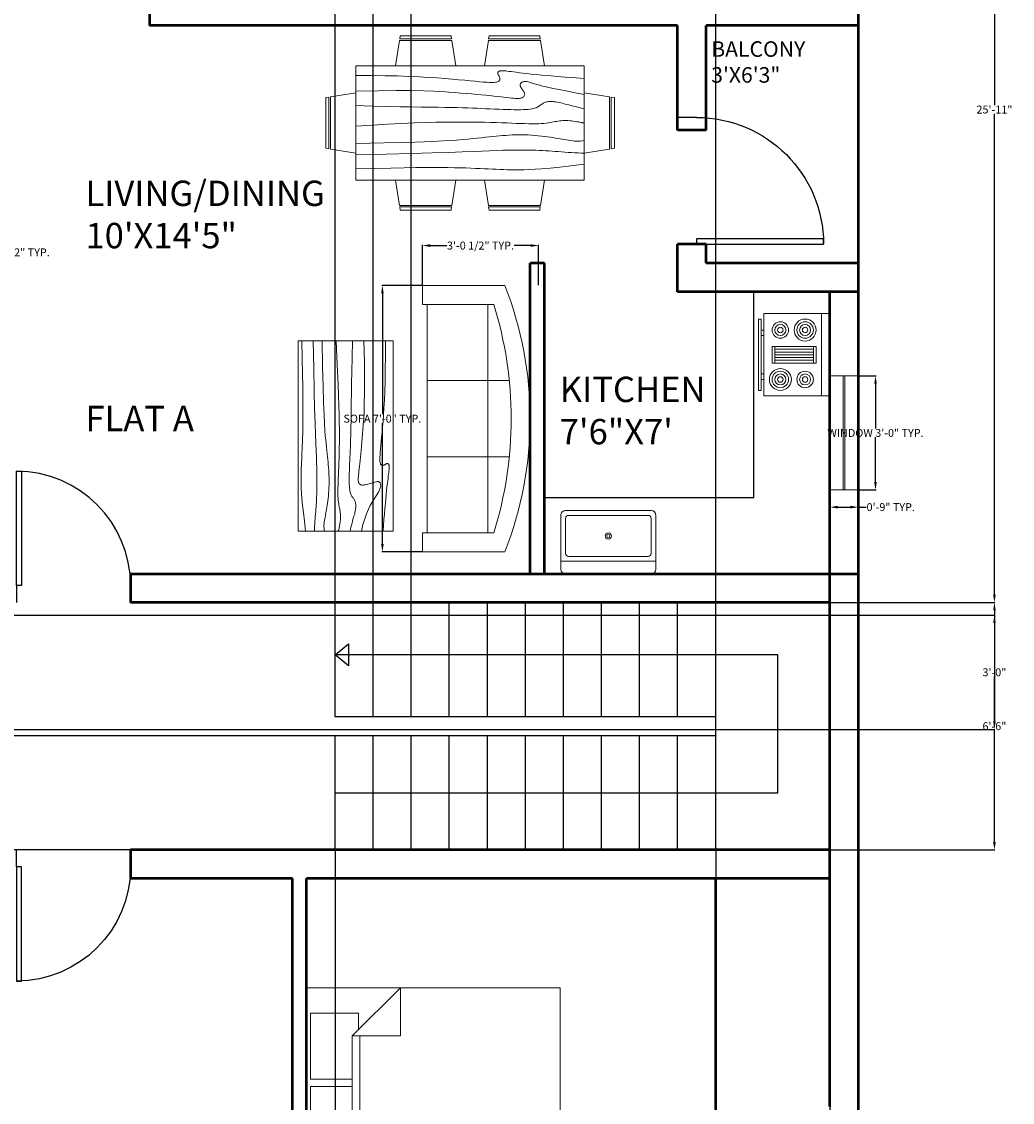
# Model space of a CAD drawing. Units: inches. Extents: x -46 to 565, y -56 to 809.
# Tile 5 of 6: x 252 to 565, y 296 to 636. Entities that reach past the tile are written whole.
import ezdxf

# ---------------------------------------------------------------- set-up
doc = ezdxf.new("R2010")
doc.units = ezdxf.units.IN
doc.header["$MEASUREMENT"] = 0
for name, color, linetype, lineweight in [('A-ANNO-DIMS', 2, 'Continuous', 18), ('A-AREA-IDEN', 241, 'Continuous', 18), ('A-FLOR-CASE', 8, 'Continuous', 25), ('A-FLOR-FIXT', 131, 'Continuous', 18), ('A-FURN', 131, 'Continuous', 18), ('DOOR', 210, 'Continuous', 25), ('EQUIPMENT', 131, 'Continuous', 18), ('STAIRCASE', 90, 'Continuous', 25), ('WALL', 10, 'Continuous', 50), ('WINDOW', 170, 'Continuous', 18)]:
    doc.layers.add(name, color=color, linetype=linetype, lineweight=lineweight)
doc.styles.get("Standard").update_dxf_attribs({"font": 'arial.ttf'})
doc.dimstyles.get("Standard").update_dxf_attribs({"dimtxt": 2.5, "dimasz": 2.5, "dimexe": 0.18, "dimexo": 0.0625, "dimgap": 0.09, "dimtad": 0, "dimtih": 1, "dimtoh": 1, "dimzin": 0, "dimdsep": 46, "dimlunit": 3, "dimtxsty": 'Standard', "dimcen": 0.09, "dimadec": 0, "dimazin": 0, "dimtfac": 1, "dimtofl": 0, "dimtmove": 0, "dimatfit": 3, "dimfxl": 1, "dimtolj": 1, "dimtzin": 0, "dimarcsym": 0})

# ---------------------------------------------------------------- blocks, each defined once
blk = doc.blocks.new('*U2')
for p, q in [((0, 0), (0, -6)), ((40, 0), (40, -6))]:
    blk.add_line(p, q)
blk.add_lwpolyline([(0, 0), (0, 40), (1.75, 40), (1.75, 0)], close=True)
blk.add_arc((0, 0), 40, 0, 90)
blk = doc.blocks.new('Table - Rectangular Woodgrain 60 x 30 in.')
for p, q in [((0, 0), (0, -30)), ((60, 0), (0, 0)), ((60, -30), (60, 0)), ((0, -30), (60, -30))]:
    blk.add_line(p, q)
for points in [[(0, -2.4), (4.8155, -2.418), (9.0302, -2.4688), (12.709, -2.5477), (15.9167, -2.65), (18.7181, -2.7711), (21.1781, -2.9063), (23.3616, -3.0508), (25.3333, -3.2), (27.1477, -3.3495), (28.8172, -3.4958), (30.3437, -3.636), (31.7291, -3.7667), (32.9756, -3.8849), (34.0849, -3.9875), (35.059, -4.0714), (35.9, -4.1334), (36.6114, -4.1711), (37.2041, -4.1854), (37.6906, -4.1779), (38.0833, -4.15), (38.3948, -4.1034), (38.6375, -4.0396), (38.8239, -3.9602), (38.9666, -3.8667), (39.0764, -3.7608), (39.1573, -3.6448), (39.2116, -3.521), (39.2416, -3.3917), (39.2498, -3.2593), (39.2385, -3.1261), (39.21, -2.9944), (39.1666, -2.8667), (39.111, -2.7447), (39.0468, -2.6281), (38.978, -2.5163), (38.9083, -2.4083), (38.8418, -2.3035), (38.7823, -2.201), (38.7337, -2.1001), (38.7, -2), (38.6844, -1.9003), (38.6875, -1.8021), (38.7094, -1.707), (38.75, -1.6167), (38.8094, -1.5326), (38.8875, -1.4563), (38.9844, -1.3893), (39.1, -1.3333), (39.2351, -1.2896), (39.3937, -1.2583), (39.5804, -1.2396), (39.8, -1.2333), (40.057, -1.2396), (40.3562, -1.2583), (40.7023, -1.2896), (41.1, -1.3333), (41.5547, -1.3895), (42.0755, -1.4573), (42.6721, -1.5361), (43.3542, -1.625), (44.1316, -1.7233), (45.014, -1.8302), (46.0114, -1.9449), (47.1333, -2.0667), (48.3862, -2.1947), (49.7625, -2.3281), (51.2513, -2.4663), (52.8416, -2.6083), (54.5226, -2.7535), (56.2833, -2.9011), (58.1127, -3.0501), (60, -3.2)], [(0, -9.2), (6.5759, -9.0858), (11.9385, -9.0365), (16.2527, -9.0418), (19.6833, -9.0917), (22.3952, -9.1759), (24.5531, -9.2844), (26.322, -9.4069), (27.8666, -9.5333), (29.3241, -9.6553), (30.7203, -9.7719), (32.0532, -9.8837), (33.3208, -9.9917), (34.5213, -10.0965), (35.6526, -10.199), (36.7128, -10.2999), (37.7, -10.4), (38.6129, -10.4996), (39.4531, -10.5969), (40.223, -10.6895), (40.925, -10.775), (41.5613, -10.8512), (42.1344, -10.9156), (42.6465, -10.966), (43.1, -11), (43.4976, -11.0158), (43.8437, -11.0136), (44.143, -10.9942), (44.4, -10.9583), (44.6195, -10.9069), (44.8062, -10.8406), (44.9648, -10.7603), (45.1, -10.6667), (45.2155, -10.5598), (45.3114, -10.4365), (45.3871, -10.2929), (45.4416, -10.125), (45.4743, -9.929), (45.4844, -9.7011), (45.4709, -9.4371), (45.4333, -9.1333), (45.3716, -8.7883), (45.2896, -8.4104), (45.1919, -8.0107), (45.0833, -7.6), (44.9685, -7.1893), (44.8521, -6.7896), (44.7388, -6.4117), (44.6333, -6.0667), (44.54, -5.7628), (44.4614, -5.4979), (44.4001, -5.2675), (44.3583, -5.0667), (44.3384, -4.8909), (44.3427, -4.7354), (44.3736, -4.5956), (44.4333, -4.4667), (44.5236, -4.3453), (44.6427, -4.2333), (44.7884, -4.1339), (44.9583, -4.05), (45.1501, -3.9849), (45.3614, -3.9417), (45.59, -3.9234), (45.8333, -3.9333), (46.0915, -3.9749), (46.3734, -4.0531), (46.6906, -4.1736), (47.0542, -4.3417), (47.4756, -4.5629), (47.9661, -4.8427), (48.5372, -5.1866), (49.2, -5.6), (49.9676, -6.0844), (50.8594, -6.625), (51.8965, -7.2031), (53.1, -7.8), (54.491, -8.3969), (56.0906, -8.975), (57.9199, -9.5156), (60, -10)], [(0, -12.8), (5.1847, -12.9322), (9.6213, -13.0323), (13.3963, -13.1059), (16.5958, -13.1583), (19.3063, -13.1952), (21.614, -13.2219), (23.6054, -13.2439), (25.3666, -13.2667), (26.9728, -13.2947), (28.4531, -13.3281), (29.8256, -13.3663), (31.1083, -13.4083), (32.3191, -13.4535), (33.476, -13.501), (34.597, -13.5501), (35.7, -13.6), (36.7984, -13.6497), (37.8875, -13.6979), (38.9578, -13.743), (40, -13.7833), (41.0047, -13.8174), (41.9625, -13.8438), (42.864, -13.8607), (43.7, -13.8667), (44.4631, -13.8604), (45.1552, -13.8417), (45.7801, -13.8104), (46.3416, -13.7667), (46.8439, -13.7104), (47.2906, -13.6417), (47.6858, -13.5604), (48.0333, -13.4667), (48.3375, -13.3608), (48.6042, -13.2448), (48.8396, -13.121), (49.05, -12.9917), (49.2417, -12.8593), (49.4208, -12.7261), (49.5937, -12.5944), (49.7667, -12.4667), (49.9452, -12.3451), (50.1323, -12.2313), (50.3303, -12.1268), (50.5416, -12.0333), (50.7686, -11.9524), (51.0135, -11.8854), (51.2788, -11.8341), (51.5666, -11.8), (51.8785, -11.7843), (52.2116, -11.7865), (52.562, -11.8059), (52.926, -11.8417), (53.2998, -11.8931), (53.6795, -11.9594), (54.0614, -12.0397), (54.4416, -12.1333), (54.8223, -12.2401), (55.2293, -12.3625), (55.6942, -12.5037), (56.2489, -12.6667), (56.9251, -12.8547), (57.7545, -13.0708), (58.7689, -13.3182), (60, -13.6)], [(0, -18), (5.124, -17.7273), (9.6609, -17.5057), (13.6705, -17.3303), (17.2125, -17.1958), (20.3467, -17.0973), (23.1328, -17.0297), (25.6307, -16.9878), (27.9, -16.9667), (29.9928, -16.9617), (31.9302, -16.9703), (33.7254, -16.9907), (35.3917, -17.0208), (36.9423, -17.0588), (38.3906, -17.1026), (39.7499, -17.1503), (41.0333, -17.2), (42.2519, -17.2496), (43.4073, -17.2969), (44.4986, -17.3395), (45.525, -17.375), (46.4858, -17.4012), (47.3802, -17.4156), (48.2074, -17.416), (48.9667, -17.4), (49.6583, -17.3662), (50.2872, -17.3167), (50.8595, -17.2547), (51.3812, -17.1833), (51.8584, -17.1057), (52.2971, -17.025), (52.7034, -16.9443), (53.0833, -16.8667), (53.443, -16.7951), (53.789, -16.7313), (54.128, -16.6768), (54.4666, -16.6334), (54.8115, -16.6024), (55.1693, -16.5854), (55.5465, -16.5841), (55.95, -16.6), (56.3828, -16.6337), (56.8346, -16.6823), (57.2915, -16.7418), (57.7396, -16.8084), (58.165, -16.878), (58.5539, -16.9469), (58.8924, -17.0111), (59.1666, -17.0667), (59.3679, -17.1107), (59.5078, -17.1438), (59.6032, -17.1675), (59.6708, -17.1833), (59.7275, -17.193), (59.7901, -17.1979), (59.8753, -17.1998), (60, -17.2)], [(0, -22.4), (8.0098, -22.2501), (14.4094, -22.1011), (19.4168, -21.9535), (23.25, -21.8083), (26.1269, -21.6663), (28.2656, -21.5281), (29.884, -21.3947), (31.2, -21.2667), (32.3967, -21.1448), (33.5172, -21.0292), (34.5697, -20.9198), (35.5625, -20.8167), (36.5037, -20.7198), (37.4015, -20.6292), (38.2642, -20.5448), (39.1, -20.4667), (39.9164, -20.3951), (40.7187, -20.3313), (41.5117, -20.2768), (42.3, -20.2333), (43.0883, -20.2024), (43.8812, -20.1854), (44.6836, -20.1841), (45.5, -20.2), (46.3328, -20.234), (47.1747, -20.2844), (48.0163, -20.3488), (48.8479, -20.425), (49.66, -20.5106), (50.4429, -20.6031), (51.1872, -20.7004), (51.8833, -20.8), (52.5246, -20.8999), (53.1166, -20.9995), (53.6681, -21.0983), (54.1875, -21.1958), (54.6834, -21.2919), (55.1646, -21.3859), (55.6394, -21.4777), (56.1167, -21.5667), (56.6028, -21.6515), (57.0961, -21.7266), (57.5929, -21.7852), (58.0896, -21.8208), (58.5823, -21.8268), (59.0674, -21.7964), (59.5412, -21.723), (60, -21.6)], [(0, -25.2), (8.6355, -25.0504), (15.7026, -24.9031), (21.4049, -24.7606), (25.9458, -24.625), (29.529, -24.4988), (32.3578, -24.3844), (34.6359, -24.284), (36.5667, -24.2), (38.3213, -24.1341), (39.9417, -24.0854), (41.437, -24.0523), (42.8167, -24.0333), (44.0901, -24.0268), (45.2667, -24.0313), (46.3557, -24.0451), (47.3667, -24.0667), (48.309, -24.0947), (49.1928, -24.1287), (50.0284, -24.168), (50.826, -24.2125), (51.5959, -24.2617), (52.3483, -24.3151), (53.0935, -24.3725), (53.8417, -24.4334), (54.6009, -24.497), (55.3699, -24.561), (56.1454, -24.6226), (56.9239, -24.6792), (57.7021, -24.7279), (58.4764, -24.7662), (59.2435, -24.7911), (60, -24.8)], [(0, -28.8), (5.6867, -28.6681), (10.45, -28.5698), (14.407, -28.5012), (17.675, -28.4584), (20.3711, -28.4374), (22.6125, -28.4344), (24.5164, -28.4455), (26.2, -28.4667), (27.762, -28.4947), (29.2276, -28.5281), (30.6033, -28.5663), (31.8958, -28.6084), (33.1118, -28.6535), (34.2578, -28.7011), (35.3405, -28.7501), (36.3666, -28.8), (37.3443, -28.8497), (38.288, -28.8974), (39.2137, -28.9412), (40.1375, -28.9792), (41.0753, -29.0093), (42.0432, -29.0297), (43.0572, -29.0384), (44.1333, -29.0333), (45.2936, -29.0114), (46.5843, -28.9641), (48.0579, -28.8816), (49.7666, -28.7542), (51.7629, -28.5721), (54.0989, -28.3255), (56.8272, -28.0048), (60, -27.6)]]:
    blk.add_lwpolyline(points)
blk = doc.blocks.new('Sofa - Roundback 7 ft.')
for p, q in [((-12.00002, -32.4421), (-12.00003, -6.5971)), ((11.99997, -32.4421), (11.99998, -6.5971)), ((-36.000027, -34), (-36.000027, -11.4696)), ((-35.999844, -13.3819), (35.9998, -13.3819)), ((35.99998, -34), (35.99998, -11.4696)), ((-36.000027, -32.4421), (35.99998, -32.4421))]:
    blk.add_line(p, q)
for points in [[(-36.000027, -34), (-42.000027, -34), (-42.000027, -8)], [(41.99998, -8), (41.99998, -34), (35.99998, -34)]]:
    blk.add_lwpolyline(points)
for centre, radius, start, end in [((0, -114.25), 114.25, 68.43141, 111.5686), ((-0.00001, -127.1968), 121.1968, 72.72033, 107.2797)]:
    blk.add_arc(centre, radius, start, end)
blk = doc.blocks.new('Bed - Queen')
for p, q in [((0, -80.00003), (0, 0)), ((0, 0), (59.99999, 0)), ((59.99999, 0), (59.99999, -80.00003)), ((7.99999, -1.2), (28.79998, -1.2)), ((7.99999, -14.4), (7.99999, -1.2)), ((28.79998, -1.2), (28.79998, -14.4)), ((31.19999, -1.2), (51.99999, -1.2)), ((31.19999, -14.4), (31.19999, -1.2)), ((51.99999, -1.2), (51.99999, -16.4)), ((0, -14.4), (44.8, -14.4)), ((44.8, -16.8), (0, -16.8)), ((59.99999, -29.6), (44.8, -14.4)), ((44.8, -14.4), (44.8, -29.6)), ((51.99999, -16.4), (46.79936, -16.4)), ((44.8, -29.6), (59.99999, -29.6)), ((59.99999, -80.00003), (0, -80.00003))]:
    blk.add_line(p, q)
blk = doc.blocks.new('Dining Set - 36 x 72 in.')
for p, q in [((-22, 27.5), (-22.1562, 26.50042)), ((-22, 27.5), (-6, 27.5)), ((-5.8437, 26.49966), (-6, 27.5)), ((6, 27.5), (5.8438, 26.50042)), ((6, 27.5), (22, 27.5)), ((22.1563, 26.49966), (22, 27.5)), ((-22.2343, 26.00059), (-23.4847, 17.99762)), ((-22.2304, 26), (-5.7608, 26)), ((-5.8416, 26.5), (-22.1534, 26.5)), ((-4.5152, 17.99762), (-5.7655, 25.99926)), ((5.7657, 26.00059), (4.5153, 17.99762)), ((5.7696, 26), (22.2392, 26)), ((22.1584, 26.5), (5.8466, 26.5)), ((23.4848, 17.99762), (22.2345, 25.99926)), ((36, 18), (-36, 18)), ((-36, 18), (-36, -18)), ((36, -18), (36, 18)), ((-45.5, 8), (-44.5004, 8.15617)), ((-45.5, 8), (-45.5, -8)), ((-44.5, -8.15843), (-44.5, 8.15338)), ((-44.0006, 8.23428), (-35.9976, 9.48474)), ((-44, 8.23041), (-44, -8.23915)), ((44.0006, 8.23428), (35.9976, 9.48474)), ((44, 8.23041), (44, -8.23915)), ((44.5, -8.15843), (44.5, 8.15338)), ((45.5, 8), (44.5005, 8.15617)), ((45.5, 8), (45.5, -8)), ((-44.4997, -8.15631), (-45.5, -8)), ((-35.9976, -9.48476), (-43.9993, -8.2345)), ((35.9976, -9.48476), (43.9993, -8.2345)), ((44.4997, -8.15631), (45.5, -8)), ((-36, -18), (36, -18)), ((-22.2343, -26.0006), (-23.4847, -17.99762)), ((-4.5152, -17.99762), (-5.7655, -25.99928)), ((5.7657, -26.0006), (4.5153, -17.99762)), ((23.4848, -17.99762), (22.2345, -25.99928)), ((-22.2304, -26), (-5.7608, -26)), ((-22, -27.5), (-22.1562, -26.50044)), ((-5.8416, -26.5), (-22.1534, -26.5)), ((-5.8437, -26.49967), (-6, -27.5)), ((5.7696, -26), (22.2392, -26)), ((6, -27.5), (5.8438, -26.50044)), ((22.1584, -26.5), (5.8466, -26.5)), ((22.1563, -26.49967), (22, -27.5)), ((-22, -27.5), (-6, -27.5)), ((6, -27.5), (22, -27.5))]:
    blk.add_line(p, q)
for points in [[(-36, 15), (-31.1772, 14.97754), (-26.8079, 14.91406), (-22.8538, 14.81543), (-19.276, 14.6875), (-16.0362, 14.53613), (-13.0957, 14.36718), (-10.4159, 14.18652), (-7.9583, 14), (-5.6904, 13.81315), (-3.6035, 13.63021), (-1.6954, 13.45508), (0.0365, 13.29166), (1.5945, 13.14388), (2.9811, 13.01562), (4.1988, 12.9108), (5.25, 12.83333), (6.1393, 12.78613), (6.8802, 12.76823), (7.4883, 12.77767), (7.9792, 12.8125), (8.3685, 12.87077), (8.6719, 12.95052), (8.9049, 13.0498), (9.0833, 13.16666), (9.2205, 13.29899), (9.3216, 13.44401), (9.3895, 13.59879), (9.4271, 13.76041), (9.4373, 13.92594), (9.4232, 14.09245), (9.3875, 14.257), (9.3333, 14.41666), (9.2638, 14.56917), (9.1836, 14.71484), (9.0975, 14.85465), (9.0104, 14.98958), (8.9272, 15.1206), (8.8529, 15.2487), (8.7922, 15.37483), (8.75, 15.5), (8.7305, 15.62467), (8.7344, 15.74739), (8.7617, 15.86621), (8.8125, 15.97916), (8.8867, 16.08431), (8.9844, 16.17968), (9.1055, 16.26334), (9.25, 16.33333), (9.4189, 16.38802), (9.6172, 16.42708), (9.8506, 16.45052), (10.125, 16.45833), (10.4463, 16.45052), (10.8203, 16.42708), (11.2529, 16.38802), (11.75, 16.33333), (12.3184, 16.26318), (12.9694, 16.17838), (13.7151, 16.07991), (14.5677, 15.96875), (15.5395, 15.84586), (16.6426, 15.71224), (17.8893, 15.56884), (19.2917, 15.41666), (20.859, 15.25667), (22.5879, 15.08984), (24.4721, 14.91715), (26.5052, 14.73958), (28.6809, 14.5581), (30.9929, 14.3737), (33.4347, 14.18733), (36, 14)], [(-36, 10), (-28.9766, 10.14274), (-23.1725, 10.20442), (-18.4241, 10.19775), (-14.5677, 10.13541), (-11.4399, 10.03011), (-8.877, 9.89453), (-6.7154, 9.74137), (-4.7917, 9.58333), (-2.9698, 9.43082), (-1.2246, 9.28515), (0.4415, 9.14534), (2.026, 9.01041), (3.5266, 8.87939), (4.9408, 8.7513), (6.266, 8.62516), (7.5, 8.5), (8.6411, 8.37549), (9.6914, 8.2539), (10.6538, 8.13818), (11.5312, 8.03125), (12.3267, 7.93603), (13.043, 7.85547), (13.6831, 7.79248), (14.25, 7.75), (14.7471, 7.7303), (15.1797, 7.73307), (15.5537, 7.75732), (15.875, 7.80208), (16.1494, 7.86637), (16.3828, 7.94922), (16.5811, 8.04964), (16.75, 8.16666), (16.8944, 8.29915), (17.0143, 8.44531), (17.1089, 8.60319), (17.1771, 8.77083), (17.218, 8.94629), (17.2305, 9.1276), (17.2137, 9.31282), (17.1667, 9.5), (17.0895, 9.6875), (16.987, 9.875), (16.8649, 10.0625), (16.7292, 10.25), (16.5856, 10.4375), (16.4401, 10.625), (16.2985, 10.8125), (16.1667, 11), (16.05, 11.18733), (15.9518, 11.3737), (15.8752, 11.5581), (15.8229, 11.73958), (15.798, 11.91715), (15.8034, 12.08984), (15.842, 12.25667), (15.9167, 12.41666), (16.0295, 12.56836), (16.1784, 12.70833), (16.3605, 12.83268), (16.5729, 12.9375), (16.8127, 13.01888), (17.0768, 13.07291), (17.3625, 13.0957), (17.6667, 13.08333), (17.9894, 13.03312), (18.3418, 12.94726), (18.7382, 12.82918), (19.1927, 12.68229), (19.7195, 12.51001), (20.3327, 12.31575), (21.0465, 12.10294), (21.875, 11.875), (22.8357, 11.63354), (23.959, 11.37304), (25.2786, 11.08618), (26.8282, 10.76562), (28.6414, 10.40405), (30.752, 9.99414), (33.1936, 9.52856), (36, 9)], [(-36, 5.5), (-30.7157, 5.3348), (-26.069, 5.20963), (-21.9946, 5.11767), (-18.4271, 5.05208), (-15.3009, 5.00602), (-12.5508, 4.97265), (-10.1112, 4.94515), (-7.9167, 4.91666), (-5.909, 4.88167), (-4.0586, 4.83984), (-2.3429, 4.79215), (-0.7396, 4.73958), (0.7739, 4.6831), (2.22, 4.6237), (3.6213, 4.56233), (5, 4.5), (6.373, 4.43782), (7.7344, 4.3776), (9.0723, 4.32129), (10.375, 4.27083), (11.6309, 4.22819), (12.8281, 4.19531), (13.9551, 4.17415), (15, 4.16666), (15.954, 4.17448), (16.819, 4.19791), (17.6001, 4.23698), (18.3021, 4.29166), (18.9299, 4.36198), (19.4883, 4.44791), (19.9823, 4.54948), (20.4167, 4.66666), (20.7969, 4.79899), (21.1302, 4.94401), (21.4245, 5.09879), (21.6875, 5.26041), (21.9271, 5.42594), (22.1511, 5.59245), (22.3672, 5.757), (22.5834, 5.91666), (22.8065, 6.06868), (23.0404, 6.21093), (23.2879, 6.34147), (23.5521, 6.45833), (23.8358, 6.55957), (24.142, 6.64323), (24.4735, 6.70735), (24.8334, 6.75), (25.2235, 6.76969), (25.642, 6.76692), (26.0858, 6.74267), (26.5521, 6.69791), (27.0379, 6.63362), (27.5404, 6.55078), (28.0565, 6.45036), (28.5834, 6.33333), (29.1242, 6.19987), (29.7071, 6.04687), (30.3661, 5.87044), (31.1354, 5.66666), (32.0493, 5.43164), (33.142, 5.16146), (34.4475, 4.85221), (36, 4.5)], [(-36, -1), (-30.7915, -0.6591), (-26.0195, -0.38216), (-21.6519, -0.16284), (-17.6563, 0.00521), (-14.0005, 0.12833), (-10.6523, 0.21289), (-7.5796, 0.26522), (-4.75, 0.29166), (-2.134, 0.29793), (0.2878, 0.28711), (2.5317, 0.26163), (4.6146, 0.22396), (6.5529, 0.17651), (8.3633, 0.12174), (10.0623, 0.06209), (11.6667, 0), (13.1899, -0.06201), (14.6341, -0.1211), (15.9982, -0.17432), (17.2813, -0.21875), (18.4823, -0.25147), (19.6003, -0.26953), (20.6343, -0.27002), (21.5834, -0.25), (22.4481, -0.20768), (23.2357, -0.14584), (23.9549, -0.06836), (24.6146, 0.02083), (25.2235, 0.11784), (25.7904, 0.21875), (26.3241, 0.31966), (26.8334, 0.41666), (27.3265, 0.50618), (27.8099, 0.58593), (28.2894, 0.65397), (28.7709, 0.70833), (29.2601, 0.74707), (29.763, 0.76823), (30.2855, 0.76985), (30.8334, 0.75), (31.4088, 0.70784), (31.9994, 0.64713), (32.589, 0.57275), (33.1615, 0.48958), (33.7008, 0.4025), (34.1908, 0.3164), (34.6153, 0.23616), (34.9584, 0.16666), (35.2099, 0.11165), (35.3848, 0.07031), (35.504, 0.04069), (35.5886, 0.02083), (35.6594, 0.00879), (35.7377, 0.0026), (35.8442, 0.00032), (36, 0)], [(-36, -6.5), (-27.1843, -6.31267), (-20.084, -6.1263), (-14.469, -5.9419), (-10.1094, -5.76042), (-6.7752, -5.58285), (-4.2363, -5.41016), (-2.2629, -5.24333), (-0.625, -5.08334), (0.8708, -4.93099), (2.2715, -4.78646), (3.5872, -4.64974), (4.8281, -4.52084), (6.0046, -4.39974), (7.127, -4.28646), (8.2053, -4.18099), (9.25, -4.08334), (10.2705, -3.99382), (11.2734, -3.91407), (12.2647, -3.84603), (13.25, -3.79167), (14.2354, -3.75293), (15.2266, -3.73177), (16.2295, -3.73015), (17.25, -3.75), (18.2912, -3.79248), (19.3451, -3.85547), (20.4009, -3.93604), (21.4479, -4.03125), (22.4754, -4.13819), (23.4727, -4.25391), (24.4289, -4.37549), (25.3334, -4.5), (26.1785, -4.62492), (26.9694, -4.74935), (27.7145, -4.87281), (28.4219, -4.99479), (29.1, -5.11483), (29.7572, -5.23242), (30.4016, -5.34709), (31.0417, -5.45834), (31.6837, -5.56437), (32.3262, -5.65821), (32.9658, -5.73153), (33.599, -5.77604), (34.2224, -5.78345), (34.8327, -5.74545), (35.4264, -5.65373), (36, -5.5)], [(-36, -10), (-26.4022, -9.81299), (-18.4675, -9.62891), (-11.9839, -9.45069), (-6.7396, -9.28125), (-2.5226, -9.12354), (0.8789, -8.98047), (3.6769, -8.85498), (6.0833, -8.75), (8.2767, -8.66765), (10.3021, -8.60677), (12.1712, -8.56543), (13.8958, -8.54167), (15.4876, -8.53353), (16.9583, -8.53907), (18.3197, -8.55632), (19.5834, -8.58334), (20.7616, -8.61841), (21.8685, -8.66081), (22.9188, -8.71004), (23.9271, -8.76563), (24.9081, -8.82707), (25.8763, -8.89388), (26.8465, -8.96558), (27.8334, -9.04167), (28.8474, -9.12118), (29.8828, -9.20117), (30.93, -9.27824), (31.9792, -9.34896), (33.0205, -9.40991), (34.0443, -9.45768), (35.0407, -9.48885), (36, -9.5)], [(-36, -14.5), (-30.0881, -14.33513), (-25.0332, -14.21224), (-20.7312, -14.12647), (-17.0781, -14.07292), (-13.97, -14.04671), (-11.3027, -14.04297), (-8.9724, -14.05681), (-6.875, -14.08334), (-4.9224, -14.11833), (-3.0905, -14.16016), (-1.3709, -14.20785), (0.2448, -14.26042), (1.7647, -14.3169), (3.1973, -14.3763), (4.5507, -14.43767), (5.8333, -14.5), (7.0554, -14.5621), (8.235, -14.62175), (9.3922, -14.67652), (10.5469, -14.72396), (11.7192, -14.76164), (12.929, -14.78711), (14.1965, -14.79794), (15.5417, -14.79167), (16.9933, -14.76424), (18.6152, -14.70508), (20.4804, -14.60197), (22.6615, -14.44271), (25.2312, -14.21509), (28.2624, -13.9069), (31.8277, -13.50594), (36, -13)]]:
    blk.add_lwpolyline(points)
blk = doc.blocks.new('Range-Oven - 30 in top')
for p, q in [((0, -3), (30, -3)), ((12, -6), (18, -6)), ((13, -20), (13, -6)), ((14, -6), (14, -20)), ((15, -20), (15, -6)), ((16, -6), (16, -20)), ((17, -20), (17, -6)), ((18, -20), (12, -20)), ((6, -24), (6, -25)), ((8, -25), (8, -24)), ((22, -25), (22, -24)), ((24, -24), (24, -25))]:
    blk.add_line(p, q)
for points in [[(0, -24), (0, 0), (30, 0), (30, -24)], [(12, -21), (12, -5), (18, -5), (18, -21)], [(2, -26), (2, -25), (28, -25), (28, -26)]]:
    blk.add_lwpolyline(points, close=True)
for centre, radius in [((6, -9), 4), ((6, -9), 3), ((6, -9), 2), ((24, -9), 3), ((24, -9), 2), ((6, -9), 1), ((24, -9), 1), ((6, -18), 3), ((24, -18), 4), ((24, -18), 3), ((6, -18), 2), ((6, -18), 1), ((24, -18), 2), ((24, -18), 1)]:
    blk.add_circle(centre, radius)
blk = doc.blocks.new('Sink-single - 30 in top')
blk.add_line((-15, -3.999996), (15, -3.999996))
for points in [[(-13.5, 0), (13.5, 0)], [(-15, -18.499996), (-15, -1.5)], [(15, -1.5), (15, -18.499996)], [(-13.5, -17.499996), (-13.5, -6.499996)], [(-12.5, -5.499996), (12.5, -5.499996)], [(13.5, -6.499996), (13.5, -17.499996)], [(13.5, -19.999996), (-13.5, -19.999996)], [(12.5, -18.499996), (-12.5, -18.499996)]]:
    blk.add_lwpolyline(points)
for radius in [1, 0.5]:
    blk.add_circle((0, -11.999996), radius)
for centre, radius, start, end in [((-13.5, -1.5), 1.5, 90, 180), ((13.5, -1.5), 1.5, 0, 90), ((-12.5, -6.499996), 1, 90, 180), ((12.5, -6.499996), 1, 0, 90), ((-13.5, -18.499996), 1.5, 180, 270), ((-12.5, -17.499996), 1, 180, 270), ((12.5, -17.499996), 1, 270, 0), ((13.5, -18.499996), 1.5, 270, 0)]:
    blk.add_arc(centre, radius, start, end)
blk = doc.blocks.new('WIN-36IN')
for p, q in [((4.25, 36), (4.25, 0)), ((4.75, 36), (4.75, 0))]:
    blk.add_line(p, q)
blk.add_lwpolyline([(0, 36), (0, 0), (9, 0), (9, 36)], close=True)
blk = doc.blocks.new('*D29')
at = {"layer": 'A-ANNO-DIMS', "color": 0, "lineweight": -2, "transparency": 16777216}
for p, q in [((378.58, 553.2), (365.86, 553.2)), ((366.04, 550.7), (366.04, 512.58)), ((366.04, 471.7), (366.04, 509.82)), ((378.58, 469.2), (365.86, 469.2))]:
    blk.add_line(p, q, dxfattribs=at)
at = {"layer": 'A-ANNO-DIMS', "color": 0, "transparency": 16777216}
for points in [[(365.63, 550.7), (366.46, 550.7), (366.04, 553.2)], [(365.63, 471.7), (366.46, 471.7), (366.04, 469.2)]]:
    blk.add_solid(points, dxfattribs=at)
at = {"layer": 'Defpoints', "color": 0, "transparency": 16777216}
for p in [(366.04, 553.2), (378.64, 553.2), (378.64, 469.2)]:
    blk.add_point(p, dxfattribs=at)
at = {"layer": 'A-ANNO-DIMS', "color": 0, "transparency": 16777216, "insert": (366.04, 511.2), "char_height": 2.5, "attachment_point": 5}
blk.add_mtext('\\A1;SOFA 7\'-0" TYP.', dxfattribs=at)
blk = doc.blocks.new('*D30')
at = {"layer": 'A-ANNO-DIMS', "color": 0, "lineweight": -2, "transparency": 16777216}
for p, q in [((378.64, 553.26), (378.64, 565.98)), ((415.31, 553.26), (415.31, 565.98)), ((381.14, 565.8), (386.35, 565.8)), ((412.81, 565.8), (407.6, 565.8))]:
    blk.add_line(p, q, dxfattribs=at)
at = {"layer": 'A-ANNO-DIMS', "color": 0, "transparency": 16777216}
for points in [[(381.14, 566.22), (381.14, 565.38), (378.64, 565.8)], [(412.81, 566.22), (412.81, 565.38), (415.31, 565.8)]]:
    blk.add_solid(points, dxfattribs=at)
at = {"layer": 'Defpoints', "color": 0, "transparency": 16777216}
for p in [(415.31, 565.8), (378.64, 553.2), (415.31, 553.2)]:
    blk.add_point(p, dxfattribs=at)
at = {"layer": 'A-ANNO-DIMS', "color": 0, "transparency": 16777216, "insert": (396.98, 565.8), "char_height": 2.5, "attachment_point": 5}
blk.add_mtext('\\A1;3\'-0 1/2" TYP.', dxfattribs=at)
blk = doc.blocks.new('*D36')
at = {"layer": 'A-ANNO-DIMS', "color": 0, "lineweight": -2, "transparency": 16777216}
for p, q in [((213.11, 567.5), (213.11, 563.48)), ((235.64, 567.5), (235.64, 563.48)), ((215.61, 563.66), (233.14, 563.66)), ((235.64, 563.66), (238.14, 563.66))]:
    blk.add_line(p, q, dxfattribs=at)
at = {"layer": 'A-ANNO-DIMS', "color": 0, "transparency": 16777216}
for points in [[(215.61, 564.08), (215.61, 563.24), (213.11, 563.66)], [(233.14, 564.08), (233.14, 563.24), (235.64, 563.66)]]:
    blk.add_solid(points, dxfattribs=at)
at = {"layer": 'Defpoints', "color": 0, "transparency": 16777216}
for p in [(213.11, 567.56), (235.64, 567.56), (235.64, 563.66)]:
    blk.add_point(p, dxfattribs=at)
at = {"layer": 'A-ANNO-DIMS', "color": 0, "transparency": 16777216, "insert": (249.62, 563.66), "char_height": 2.5, "attachment_point": 5}
blk.add_mtext('\\A1;1\'-10 1/2" TYP.', dxfattribs=at)
blk = doc.blocks.new('*D37')
at = {"layer": 'A-ANNO-DIMS', "color": 0, "lineweight": -2, "transparency": 16777216}
for p, q in [((516.21, 524.7), (521.72, 524.7)), ((521.54, 522.2), (521.54, 508.08)), ((521.54, 491.2), (521.54, 505.32)), ((516.21, 488.7), (521.72, 488.7))]:
    blk.add_line(p, q, dxfattribs=at)
at = {"layer": 'A-ANNO-DIMS', "color": 0, "transparency": 16777216}
for points in [[(521.13, 522.2), (521.96, 522.2), (521.54, 524.7)], [(521.13, 491.2), (521.96, 491.2), (521.54, 488.7)]]:
    blk.add_solid(points, dxfattribs=at)
at = {"layer": 'Defpoints', "color": 0, "transparency": 16777216}
for p in [(516.14, 524.7), (521.54, 524.7), (516.14, 488.7)]:
    blk.add_point(p, dxfattribs=at)
at = {"layer": 'A-ANNO-DIMS', "color": 0, "transparency": 16777216, "insert": (521.54, 506.7), "char_height": 2.5, "attachment_point": 5}
blk.add_mtext('\\A1;WINDOW 3\'-0" TYP.', dxfattribs=at)
blk = doc.blocks.new('*D38')
at = {"layer": 'A-ANNO-DIMS', "color": 0, "lineweight": -2, "transparency": 16777216}
for p, q in [((507.14, 488.64), (507.14, 483.12)), ((516.14, 488.64), (516.14, 483.12)), ((509.64, 483.3), (513.64, 483.3)), ((516.14, 483.3), (518.64, 483.3))]:
    blk.add_line(p, q, dxfattribs=at)
at = {"layer": 'A-ANNO-DIMS', "color": 0, "transparency": 16777216}
for points in [[(509.64, 483.72), (509.64, 482.88), (507.14, 483.3)], [(513.64, 483.72), (513.64, 482.88), (516.14, 483.3)]]:
    blk.add_solid(points, dxfattribs=at)
at = {"layer": 'Defpoints', "color": 0, "transparency": 16777216}
for p in [(507.14, 488.7), (516.14, 488.7), (516.14, 483.3)]:
    blk.add_point(p, dxfattribs=at)
at = {"layer": 'A-ANNO-DIMS', "color": 0, "transparency": 16777216, "insert": (526.35, 483.3), "char_height": 2.5, "attachment_point": 5}
blk.add_mtext('\\A1;0\'-9" TYP.', dxfattribs=at)
blk = doc.blocks.new('*D39')
at = {"layer": 'A-ANNO-DIMS', "color": 0, "lineweight": -2, "transparency": 16777216}
for p, q in [((516.21, 764.2), (559.22, 764.2)), ((559.04, 761.7), (559.04, 610.07)), ((559.04, 455.7), (559.04, 607.33)), ((507.21, 453.2), (559.22, 453.2))]:
    blk.add_line(p, q, dxfattribs=at)
at = {"layer": 'A-ANNO-DIMS', "color": 0, "transparency": 16777216}
for points in [[(558.63, 761.7), (559.46, 761.7), (559.04, 764.2)], [(558.63, 455.7), (559.46, 455.7), (559.04, 453.2)]]:
    blk.add_solid(points, dxfattribs=at)
at = {"layer": 'Defpoints', "color": 0, "transparency": 16777216}
for p in [(516.14, 764.2), (507.14, 453.2), (559.04, 453.2)]:
    blk.add_point(p, dxfattribs=at)
at = {"layer": 'A-ANNO-DIMS', "color": 0, "transparency": 16777216, "insert": (559.04, 608.7), "char_height": 2.5, "attachment_point": 5}
blk.add_mtext('\\A1;25\'-11"', dxfattribs=at)
blk = doc.blocks.new('*D40')
at = {"layer": 'A-ANNO-DIMS', "color": 0, "lineweight": -2, "transparency": 16777216}
for p, q in [((507.21, 453.2), (559.22, 453.2)), ((559.04, 450.7), (559.04, 415.57)), ((559.04, 377.7), (559.04, 412.83)), ((507.21, 375.2), (559.22, 375.2))]:
    blk.add_line(p, q, dxfattribs=at)
at = {"layer": 'A-ANNO-DIMS', "color": 0, "transparency": 16777216}
for points in [[(558.63, 450.7), (559.46, 450.7), (559.04, 453.2)], [(558.63, 377.7), (559.46, 377.7), (559.04, 375.2)]]:
    blk.add_solid(points, dxfattribs=at)
at = {"layer": 'Defpoints', "color": 0, "transparency": 16777216}
for p in [(507.14, 453.2), (559.04, 453.2), (507.14, 375.2)]:
    blk.add_point(p, dxfattribs=at)
at = {"layer": 'A-ANNO-DIMS', "color": 0, "transparency": 16777216, "insert": (559.04, 414.2), "char_height": 2.5, "attachment_point": 5}
blk.add_mtext('\\A1;6\'-6"', dxfattribs=at)
blk = doc.blocks.new('*D41')
at = {"layer": 'A-ANNO-DIMS', "color": 0, "lineweight": -2, "transparency": 16777216}
for p, q in [((351.14, 417.26), (351.14, 807.28)), ((353.64, 807.1), (406.88, 807.1)), ((468.64, 807.1), (415.41, 807.1)), ((471.14, 417.26), (471.14, 807.28))]:
    blk.add_line(p, q, dxfattribs=at)
at = {"layer": 'A-ANNO-DIMS', "color": 0, "transparency": 16777216}
for points in [[(353.64, 807.52), (353.64, 806.68), (351.14, 807.1)], [(468.64, 807.52), (468.64, 806.68), (471.14, 807.1)]]:
    blk.add_solid(points, dxfattribs=at)
at = {"layer": 'Defpoints', "color": 0, "transparency": 16777216}
for p in [(471.14, 807.1), (351.14, 417.2), (471.14, 417.2)]:
    blk.add_point(p, dxfattribs=at)
at = {"layer": 'A-ANNO-DIMS', "color": 0, "transparency": 16777216, "insert": (411.14, 807.1), "char_height": 2.5, "attachment_point": 5}
blk.add_mtext('\\A1;10\'-0"', dxfattribs=at)
blk = doc.blocks.new('*D42')
at = {"layer": 'A-ANNO-DIMS', "color": 0, "lineweight": -2, "transparency": 16777216}
for p, q in [((471.14, 375.14), (471.14, 0.22)), ((507.14, 375.14), (507.14, 0.22)), ((473.64, 0.4), (485.73, 0.4)), ((504.64, 0.4), (492.55, 0.4))]:
    blk.add_line(p, q, dxfattribs=at)
at = {"layer": 'A-ANNO-DIMS', "color": 0, "transparency": 16777216}
for points in [[(473.64, 0.82), (473.64, -0.02), (471.14, 0.4)], [(504.64, 0.82), (504.64, -0.02), (507.14, 0.4)]]:
    blk.add_solid(points, dxfattribs=at)
at = {"layer": 'Defpoints', "color": 0, "transparency": 16777216}
for p in [(471.14, 375.2), (507.14, 375.2), (507.14, 0.4)]:
    blk.add_point(p, dxfattribs=at)
at = {"layer": 'A-ANNO-DIMS', "color": 0, "transparency": 16777216, "insert": (489.14, 0.4), "char_height": 2.5, "attachment_point": 5}
blk.add_mtext('\\A1;3\'-0"', dxfattribs=at)
blk = doc.blocks.new('*D43')
at = {"layer": 'A-ANNO-DIMS', "color": 0, "lineweight": -2, "transparency": 16777216}
for p, q in [((244.64, 375.14), (244.64, 0.22)), ((351.14, 375.14), (351.14, 0.22)), ((247.14, 0.4), (290.59, 0.4)), ((348.64, 0.4), (305.19, 0.4))]:
    blk.add_line(p, q, dxfattribs=at)
at = {"layer": 'A-ANNO-DIMS', "color": 0, "transparency": 16777216}
for points in [[(247.14, 0.82), (247.14, -0.02), (244.64, 0.4)], [(348.64, 0.82), (348.64, -0.02), (351.14, 0.4)]]:
    blk.add_solid(points, dxfattribs=at)
at = {"layer": 'Defpoints', "color": 0, "transparency": 16777216}
for p in [(244.64, 375.2), (351.14, 375.2), (351.14, 0.4)]:
    blk.add_point(p, dxfattribs=at)
at = {"layer": 'A-ANNO-DIMS', "color": 0, "transparency": 16777216, "insert": (297.89, 0.4), "char_height": 2.5, "attachment_point": 5}
blk.add_mtext('\\A1;8\'-10 1/2"', dxfattribs=at)
blk = doc.blocks.new('*D44')
at = {"layer": 'A-ANNO-DIMS', "color": 0, "lineweight": -2, "transparency": 16777216}
for p, q in [((351.08, 411.2), (-6.94, 411.2)), ((-6.76, 408.7), (-6.76, 394.57)), ((-6.76, 377.7), (-6.76, 391.83)), ((351.08, 375.2), (-6.94, 375.2))]:
    blk.add_line(p, q, dxfattribs=at)
at = {"layer": 'A-ANNO-DIMS', "color": 0, "transparency": 16777216}
for points in [[(-7.17, 408.7), (-6.34, 408.7), (-6.76, 411.2)], [(-7.17, 377.7), (-6.34, 377.7), (-6.76, 375.2)]]:
    blk.add_solid(points, dxfattribs=at)
at = {"layer": 'Defpoints', "color": 0, "transparency": 16777216}
for p in [(-6.76, 411.2), (351.14, 411.2), (351.14, 375.2)]:
    blk.add_point(p, dxfattribs=at)
at = {"layer": 'A-ANNO-DIMS', "color": 0, "transparency": 16777216, "insert": (-6.76, 393.2), "char_height": 2.5, "attachment_point": 5}
blk.add_mtext('\\A1;3\'-0"', dxfattribs=at)
blk = doc.blocks.new('*D45')
at = {"layer": 'A-ANNO-DIMS', "color": 0, "lineweight": -2, "transparency": 16777216}
for p, q in [((363.14, 453.26), (363.14, 807.28)), ((365.64, 807.1), (365.85, 807.1)), ((372.64, 807.1), (372.44, 807.1)), ((375.14, 453.26), (375.14, 807.28))]:
    blk.add_line(p, q, dxfattribs=at)
at = {"layer": 'A-ANNO-DIMS', "color": 0, "transparency": 16777216}
for points in [[(365.64, 807.52), (365.64, 806.68), (363.14, 807.1)], [(372.64, 807.52), (372.64, 806.68), (375.14, 807.1)]]:
    blk.add_solid(points, dxfattribs=at)
at = {"layer": 'Defpoints', "color": 0, "transparency": 16777216}
for p in [(375.14, 807.1), (363.14, 453.2), (375.14, 453.2)]:
    blk.add_point(p, dxfattribs=at)
at = {"layer": 'A-ANNO-DIMS', "color": 0, "transparency": 16777216, "insert": (369.14, 807.1), "char_height": 2.5, "attachment_point": 5}
blk.add_mtext('\\A1;1\'-0"', dxfattribs=at)
blk = doc.blocks.new('*D53')
at = {"layer": 'A-ANNO-DIMS', "color": 0, "lineweight": -2, "transparency": 16777216}
for p, q in [((244.71, 449.2), (559.22, 449.2)), ((559.04, 446.7), (559.04, 432.57)), ((559.04, 415.7), (559.04, 429.83)), ((244.71, 413.2), (559.22, 413.2))]:
    blk.add_line(p, q, dxfattribs=at)
at = {"layer": 'A-ANNO-DIMS', "color": 0, "transparency": 16777216}
for points in [[(558.63, 446.7), (559.46, 446.7), (559.04, 449.2)], [(558.63, 415.7), (559.46, 415.7), (559.04, 413.2)]]:
    blk.add_solid(points, dxfattribs=at)
at = {"layer": 'Defpoints', "color": 0, "transparency": 16777216}
for p in [(244.64, 449.2), (559.04, 449.2), (244.64, 413.2)]:
    blk.add_point(p, dxfattribs=at)
at = {"layer": 'A-ANNO-DIMS', "color": 0, "transparency": 16777216, "insert": (559.04, 431.2), "char_height": 2.5, "attachment_point": 5}
blk.add_mtext('\\A1;3\'-0"', dxfattribs=at)

msp = doc.modelspace()

# ---------------------------------------------------------------- linework, layer by layer
at = {"layer": 'A-FLOR-CASE'}
for q in [(483.143, 551.2), (417.143, 486.2)]:
    msp.add_line((483.143, 486.2), q, dxfattribs=at)
at = {"layer": 'STAIRCASE'}
for p, q in [((351.143, 417.2), (351.143, 453.2)), ((363.143, 417.2), (363.143, 453.2)), ((375.143, 417.2), (375.143, 453.2)), ((387.143, 417.2), (387.143, 453.2)), ((399.143, 417.2), (399.143, 453.2)), ((411.143, 417.2), (411.143, 453.2)), ((423.143, 417.2), (423.143, 453.2)), ((435.143, 417.2), (435.143, 453.2)), ((447.143, 417.2), (447.143, 453.2)), ((459.143, 417.2), (459.143, 453.2)), ((471.143, 375.2), (471.143, 453.2)), ((351.143, 436.712), (355.304, 440.135)), ((355.304, 440.135), (355.304, 433.198)), ((490.743, 436.712), (351.143, 436.712)), ((355.304, 433.198), (351.143, 436.712)), ((490.743, 393.2), (490.743, 436.712)), ((471.143, 417.2), (351.143, 417.2)), ((471.143, 411.2), (351.143, 411.2)), ((351.143, 375.2), (351.143, 411.2)), ((363.143, 375.2), (363.143, 411.2)), ((375.143, 375.2), (375.143, 411.2)), ((387.143, 375.2), (387.143, 411.2)), ((399.143, 375.2), (399.143, 411.2)), ((411.143, 375.2), (411.143, 411.2)), ((423.143, 375.2), (423.143, 411.2)), ((435.143, 375.2), (435.143, 411.2)), ((447.143, 375.2), (447.143, 411.2)), ((459.143, 375.2), (459.143, 411.2)), ((351.143, 393.2), (490.743, 393.2))]:
    msp.add_line(p, q, dxfattribs=at)
at = {"layer": 'WALL'}
for p, q in [((292.643, 639.7), (292.643, 635.2)), ((516.143, 551.2), (516.143, 639.7)), ((459.143, 635.2), (292.643, 635.2)), ((459.143, 602.2), (459.143, 635.2)), ((516.143, 635.2), (468.143, 635.2)), ((468.143, 602.2), (468.143, 635.2)), ((468.143, 602.2), (459.143, 602.2)), ((459.143, 551.2), (459.143, 566.2)), ((468.143, 566.2), (459.143, 566.2)), ((468.143, 560.2), (468.143, 566.2)), ((412.643, 462.2), (412.643, 560.2)), ((417.143, 560.2), (412.643, 560.2)), ((417.143, 462.2), (417.143, 560.2)), ((516.143, 560.2), (468.143, 560.2)), ((516.143, 551.2), (459.143, 551.2)), ((507.143, 462.2), (507.143, 551.2)), ((516.143, 462.2), (516.143, 551.2)), ((417.143, 462.2), (286.643, 462.2)), ((286.643, 462.2), (286.643, 453.2)), ((516.143, 462.2), (417.143, 462.2)), ((507.143, 453.2), (507.143, 462.2)), ((516.143, 285.2), (516.143, 462.2)), ((507.143, 453.2), (286.643, 453.2)), ((507.143, 375.2), (507.143, 453.2)), ((507.143, 375.2), (286.643, 375.2)), ((286.643, 375.2), (286.643, 366.2)), ((507.143, 294.2), (507.143, 375.2)), ((337.643, 366.2), (286.643, 366.2)), ((337.643, 232.7), (337.643, 366.2)), ((507.143, 366.2), (342.143, 366.2)), ((342.143, 237.2), (342.143, 366.2)), ((471.143, 237.2), (471.143, 366.2))]:
    msp.add_line(p, q, dxfattribs=at)

# ---------------------------------------------------------------- block references
at = {"layer": 'A-FLOR-FIXT', "rotation": 180}
msp.add_blockref('Sink-single - 30 in top', (437.302, 462.2), dxfattribs=at)
at = {"layer": 'A-FURN'}
msp.add_blockref('Dining Set - 36 x 72 in.', (393.686, 604.474), dxfattribs=at)
at = {"layer": 'A-FURN', "xscale": -1, "rotation": 270}
msp.add_blockref('Sofa - Roundback 7 ft.', (412.643, 511.2), dxfattribs=at)
at = {"layer": 'A-FURN'}
for name, p, rotation in [('Table - Rectangular Woodgrain 60 x 30 in.', (369.432, 535.719), 270), ('Bed - Queen', (342.143, 271.7), 90)]:
    msp.add_blockref(name, p, dxfattribs=dict(at, rotation=rotation))
at = {"layer": 'DOOR', "xscale": -1, "rotation": 270}
msp.add_blockref('*U2', (465.143, 566.2), dxfattribs=at)
at = {"layer": 'DOOR', "xscale": 0.9, "yscale": 0.9, "zscale": 0.9}
msp.add_blockref('*U2', (250.643, 458.6), dxfattribs=at)
at = {"layer": 'DOOR', "xscale": -0.9000000000000007, "yscale": 0.9000000000000007, "zscale": 0.9000000000000007, "rotation": 180}
msp.add_blockref('*U2', (250.643, 369.8), dxfattribs=at)
at = {"layer": 'EQUIPMENT', "xscale": 0.8666666666666667, "yscale": 0.8666666666666667, "zscale": 0.8666666666666667, "rotation": 270}
msp.add_blockref('Range-Oven - 30 in top', (507.143, 544.355), dxfattribs=at)
at = {"layer": 'WINDOW'}
msp.add_blockref('WIN-36IN', (507.143, 488.7), dxfattribs=at)

# ---------------------------------------------------------------- texts
at = {"layer": 'A-AREA-IDEN', "attachment_point": 1}
for s, width, gutter_width, heights, insert, char_height in [('BALCONY\\P3\'X6\'3" ', 43.29968, 0.612, [0], (469.732, 630.23), 4.8946), ('LIVING/DINING\\P10\'X14\'5"', 70.77133, 1, [21.644], (272.399, 586.277), 8), ('KITCHEN\\P7\'6"X7\' ', 70.77133, 1, [0], (421.962, 524.443), 8), ('FLAT A', 70.77133, 1, [0], (272.399, 515.256), 8)]:
    msp.add_mtext_dynamic_manual_height_columns(s, width=width, gutter_width=gutter_width, heights=heights, dxfattribs=dict(at, insert=insert, char_height=char_height))

# ---------------------------------------------------------------- dimensions: what is measured, and where the dimension line sits
at = {"layer": 'A-ANNO-DIMS'}
for base, p1, p2, picture, middle in [((471.143, 807.1), (351.143, 417.2), (471.143, 417.2), '*D41', (411.143, 807.1)), ((375.143, 807.1), (363.143, 453.2), (375.143, 453.2), '*D45', (369.143, 807.1)), ((351.143, 0.4), (244.643, 375.2), (351.143, 375.2), '*D43', (297.893, 0.4)), ((507.143, 0.4), (471.143, 375.2), (507.143, 375.2), '*D42', (489.143, 0.4))]:
    dim = msp.add_linear_dim(base=base, p1=p1, p2=p2, dimstyle='Standard', override={"dimdec": 1, "dimlfac": 1, "dimrnd": 0, "dimzin": 1, "dimdsep": 46, "dimlunit": 4, "dimfrac": 2}, dxfattribs=at)
    dim.commit()
    dim.dimension.update_dxf_attribs({"geometry": picture, "text_midpoint": middle})
for base, p1, p2, picture, middle in [((559.043, 453.2), (516.143, 764.2), (507.143, 453.2), '*D39', (559.043, 608.7)), ((559.043, 453.2), (507.143, 375.2), (507.143, 453.2), '*D40', (559.043, 414.2)), ((559.043, 449.2), (244.643, 413.2), (244.643, 449.2), '*D53', (559.043, 431.2)), ((-6.757, 411.2), (351.143, 375.2), (351.143, 411.2), '*D44', (-6.757, 393.2))]:
    dim = msp.add_linear_dim(base=base, p1=p1, p2=p2, angle=90, dimstyle='Standard', override={"dimdec": 1, "dimlfac": 1, "dimrnd": 0, "dimzin": 1, "dimdsep": 46, "dimlunit": 4, "dimfrac": 2}, dxfattribs=at)
    dim.commit()
    dim.dimension.update_dxf_attribs({"geometry": picture, "text_midpoint": middle})
for base, p1, p2, picture, middle in [((235.643, 563.659), (213.11, 567.559), (235.643, 567.559), '*D36', (249.618, 563.659)), ((415.31, 565.8), (378.643, 553.2), (415.31, 553.2), '*D30', (396.976, 565.8)), ((516.143, 483.3), (507.143, 488.7), (516.143, 488.7), '*D38', (526.352, 483.3))]:
    dim = msp.add_linear_dim(base=base, p1=p1, p2=p2, text='<> TYP.', dimstyle='Standard', override={"dimdec": 1, "dimlfac": 1, "dimrnd": 0, "dimzin": 1, "dimdsep": 46, "dimlunit": 4, "dimfrac": 2}, dxfattribs=at)
    dim.commit()
    dim.dimension.update_dxf_attribs({"geometry": picture, "text_midpoint": middle})
for base, p1, p2, text, picture, middle in [((366.043, 553.2), (378.643, 469.2), (378.643, 553.2), 'SOFA <> TYP.', '*D29', (366.043, 511.2)), ((521.543, 524.7), (516.143, 488.7), (516.143, 524.7), 'WINDOW <> TYP.', '*D37', (521.543, 506.7))]:
    dim = msp.add_linear_dim(base=base, p1=p1, p2=p2, angle=90, text=text, dimstyle='Standard', override={"dimdec": 1, "dimlfac": 1, "dimrnd": 0, "dimzin": 1, "dimdsep": 46, "dimlunit": 4, "dimfrac": 2}, dxfattribs=at)
    dim.commit()
    dim.dimension.update_dxf_attribs({"geometry": picture, "text_midpoint": middle})

doc.saveas('drawing.dxf')
